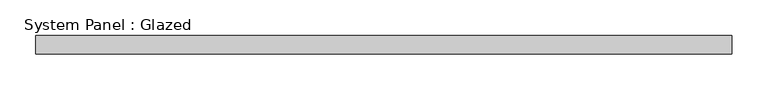
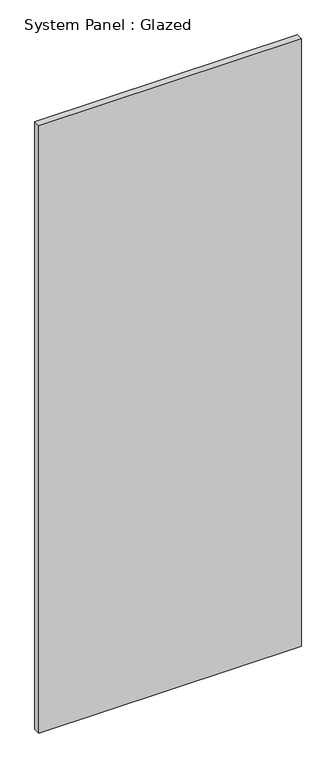
"""IFC4 building model written with IfcOpenShell, lengths in millimetres: plate geometry, System Panel : Glazed."""

from ifc_helpers import new_model, si_unit, origin, origin_with_axes, place, context, project, spatial, polyline, outline, extrude, source, transform, mapped, element, save


def system_panel_glazed_387c9df4(model_context):
    return source(origin(), model_context, "Body", "SweptSolid", [
        extrude(outline(polyline([(485.775, 19.05), (-485.775, 19.05), (-485.775, 44.45), (485.775, 44.45), (485.775, 19.05)])), origin_with_axes(), (0.0, 0.0, 1.0), 2374.9),
    ])


if __name__ == "__main__":
    model = new_model("IFC4")
    model_context = context("Model", 3, world=origin())
    ifc_project = project(units=[si_unit("LENGTHUNIT", "METRE", prefix="MILLI")], contexts=[model_context])
    site = spatial("IfcSite", under=ifc_project)
    building = spatial("IfcBuilding", under=site)
    placement = place(None, origin())
    system_panel_glazed_shape = system_panel_glazed_387c9df4(model_context)
    element("IfcPlate", 1, ObjectType="System Panel : Glazed", at=placement, inside=building, context=model_context, shape_type="MappedRepresentation", body=[
        mapped(system_panel_glazed_shape, transform((0.0, 0.0, 0.0), x_axis=(1.0, 0.0, 0.0), y_axis=(0.0, 1.0, 0.0), z_axis=(0.0, 0.0, 1.0))),
    ])
    save(model, "model.ifc")

# Revit data of these elements
# Type "System Panel : Glazed"
#   Construction Type Id = "GSP4R"
#   Analytic Construction = "1/8 in Pilkington single glazing"
#   Visual Light Transmittance = 0.9
#   Solar Heat Gain Coefficient = 0.86
#   Heat Transfer Coefficient (U) = 1.18115 BTU/(h·ft²·°F)
# Element 1 (IfcPlate, "System Panel : Glazed")
#   Materials on its faces: "Glass"
# Materials
#   "Glass": class "Glass", colour RGB 0 128 192, transparency 0.75, Description = "Soda Lime Glass", Cost = 0
